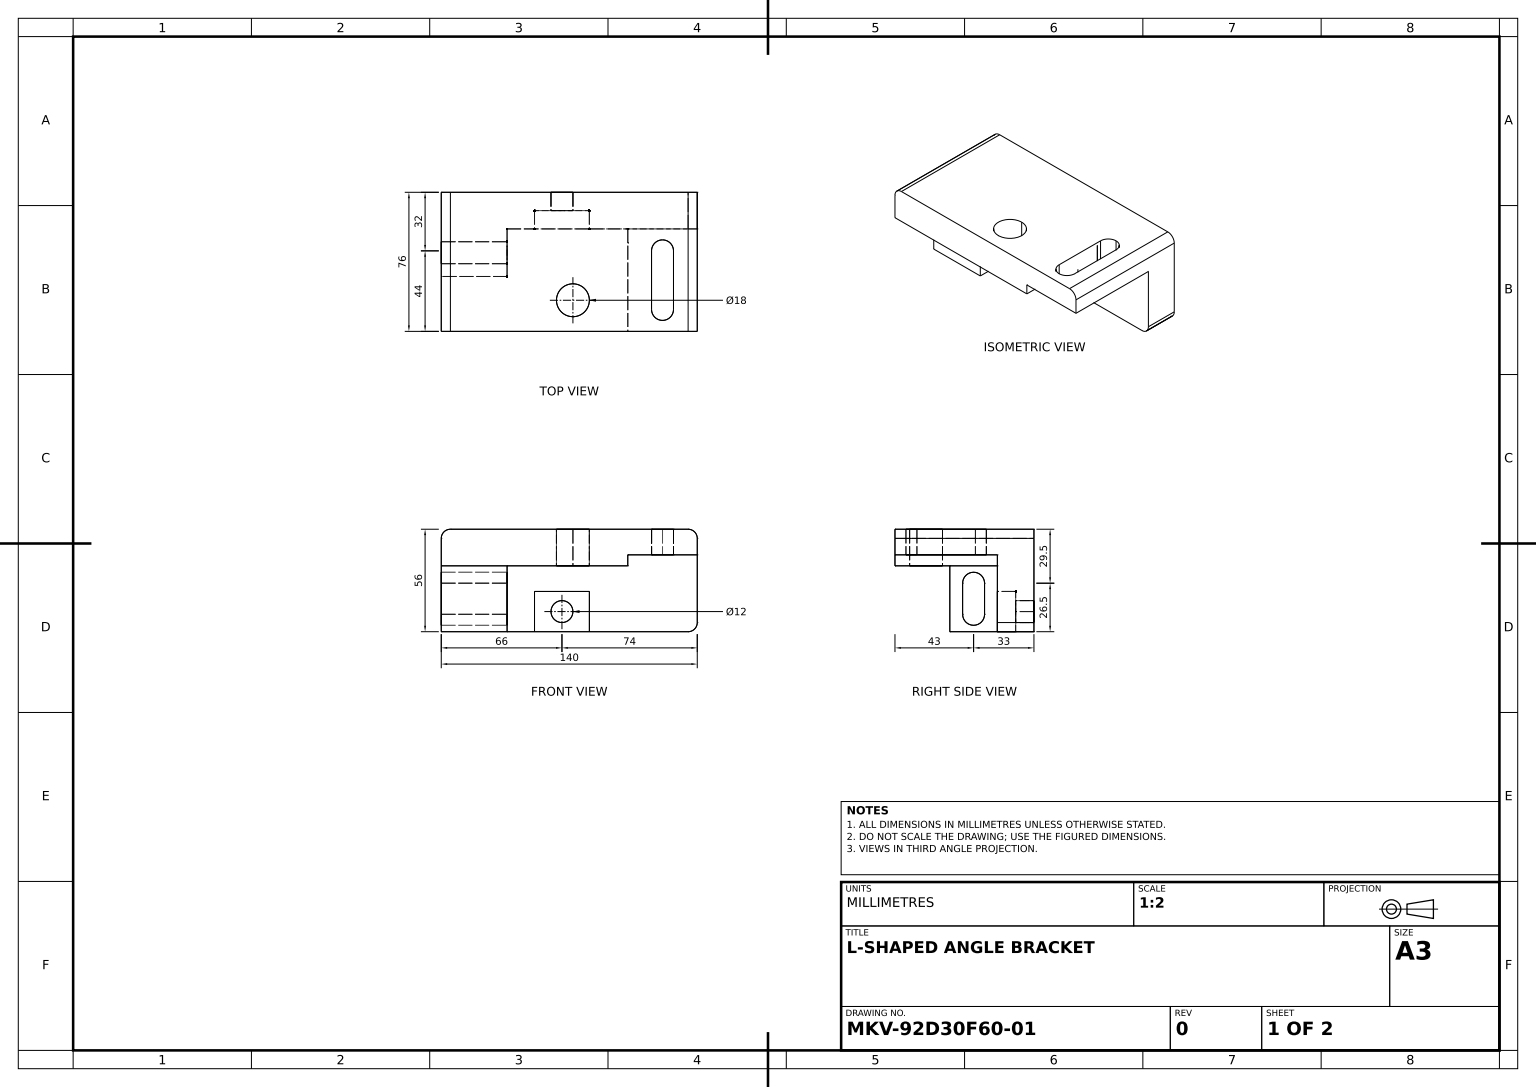
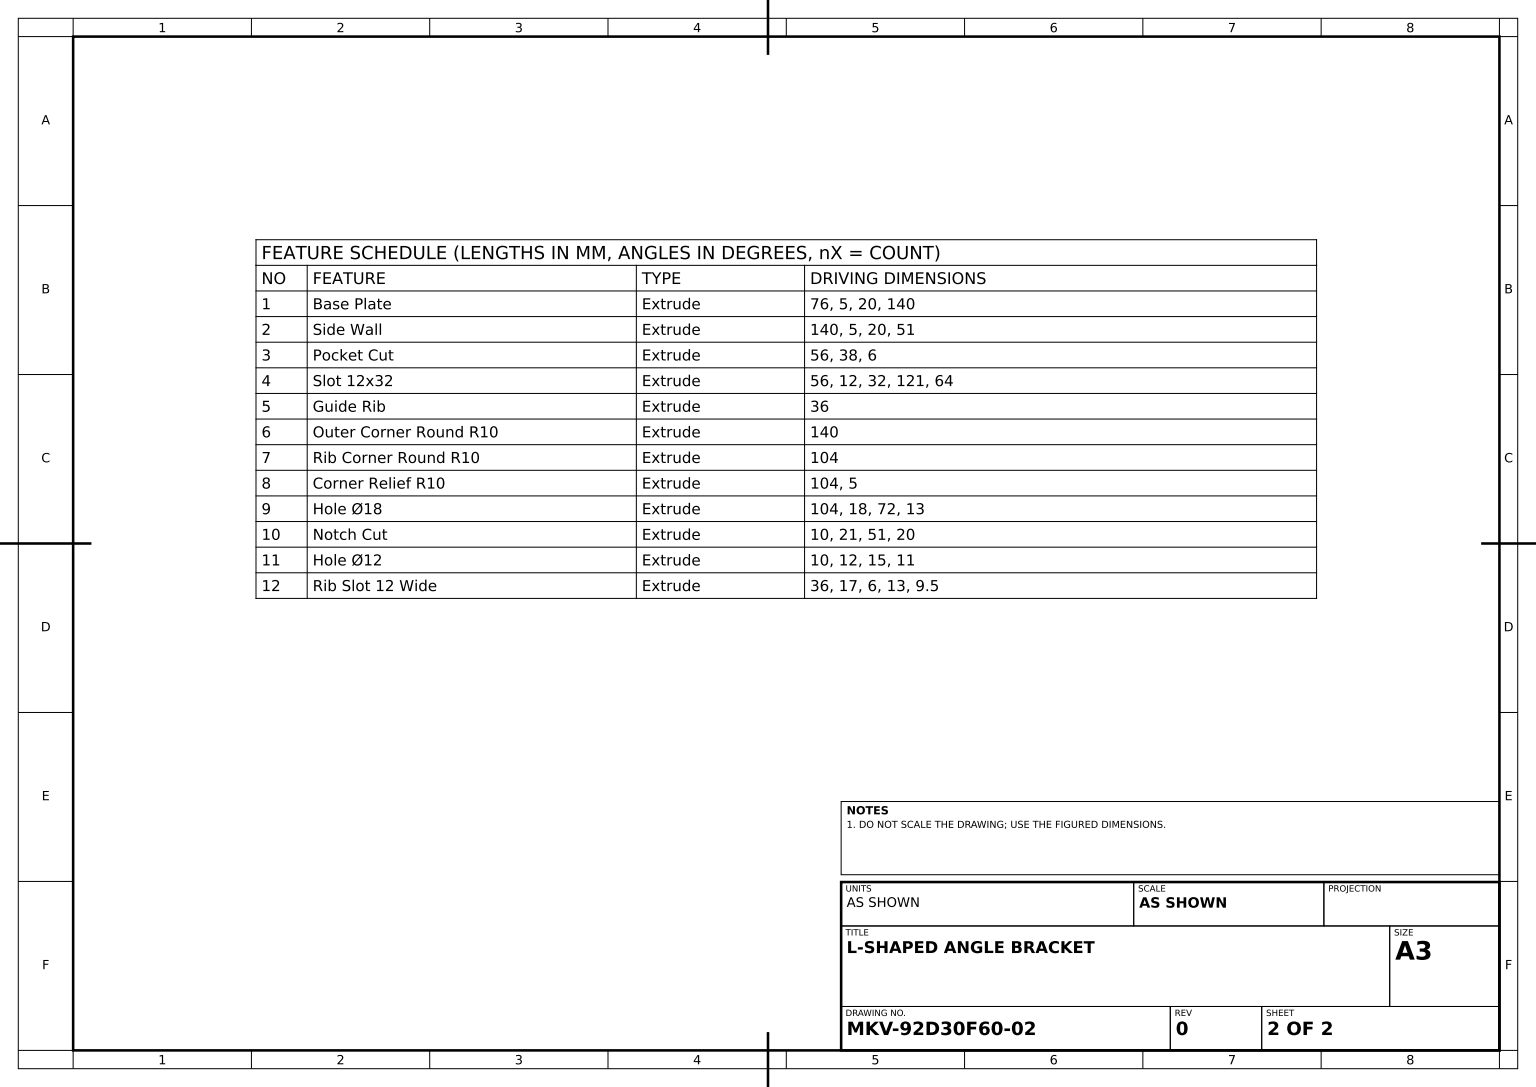
SolidWorks part; units mm, degrees
material "Plain Carbon Steel"
ref_plane "Front Plane" through (0, 0, 0) normal (0, 0, 1) x (1, 0, 0)
ref_plane "Top Plane" through (0, 0, 0) normal (0, 1, 0) x (1, 0, 0)
ref_plane "Right Plane" through (0, 0, 0) normal (1, 0, 0) x (0, 0, -1)
sketch "Base Plate Profile" plane through (0, 0, 0) normal (0, 0, 1) x (1, 0, 0)
  line L0 (5, 0) -> (135, 0)
  line L1 (140, -5) -> (140, -20)
  line L2 (140, -20) -> (0, -20)
  line L3 (0, -20) -> (0, -5)
  arc A0 (140, -5) -> (135, 0) centre (135, -5) ccw
  arc A1 (0, -5) -> (5, 0) centre (5, -5) cw
  point P9 (0, 0)
  dimension "D1" = 5
  dimension "D2" = 20
  dimension "D3" = 140
extrude "Base Plate" add sketch "Base Plate Profile" along normal blind 76
sketch "Side Wall Profile" plane through (140, 0, 0) normal (1, 0, 0) x (0, 0, -1)
  line L0 (0, -20) -> (0, -51)
  line L1 (-5, -56) -> (-15, -56)
  line L2 (-20, -51) -> (-20, -20)
  line L3 (-76, -20) -> (0, -20) construction
  line L4 (-20, -20) -> (0, -20)
  line L5 (-76, -5) -> (0, -5) construction
  arc A0 (-5, -56) -> (0, -51) centre (-5, -51) ccw
  arc A1 (-15, -56) -> (-20, -51) centre (-15, -51) cw
  dimension "D1" = 5
  dimension "D2" = 20
  dimension "D3" = 51
extrude "Side Wall" add sketch "Side Wall Profile" against normal blind 140
sketch "Pocket Profile" plane through (0, 0, 76) normal (0, 0, 1) x (1, 0, 0)
  line L0 (140, -20) -> (140, -14)
  line L1 (140, -20) -> (140, -5) construction
  line L2 (140, -14) -> (102, -14)
  line L3 (102, -14) -> (102, -20)
  line L4 (0, -20) -> (140, -20) construction
  line L5 (102, -20) -> (140, -20)
  line L6 (0, -20) -> (140, -20) construction
  dimension "D1" = 38
  dimension "D2" = 6
extrude "Pocket Cut" cut sketch "Pocket Profile" against normal blind 56
sketch "Slot 12x32 Profile" plane through (0, -14, 0) normal (0, -1, 0) x (1, 0, 0)
  line L4 (115, 64) -> (115, 32)
  line L5 (127, 64) -> (127, 32)
  arc A0 (127, 64) -> (115, 64) centre (121, 64) ccw
  arc A1 (115, 32) -> (127, 32) centre (121, 32) ccw
  dimension "D1" = 12
  dimension "D2" = 12
  dimension "D3" = 32
  dimension "D4" = 121
  dimension "D5" = 64
extrude "Slot 12x32" cut sketch "Slot 12x32 Profile" against normal blind 56
sketch "Guide Rib Profile" plane through (0, 0, 0) normal (-1, 0, 0) x (0, 0, 1)
  line L0 (20, -20) -> (46, -20)
  line L1 (76, -20) -> (20, -20) construction
  line L2 (46, -20) -> (46, -56)
  line L3 (46, -56) -> (15, -56)
  line L4 (20, -20) -> (20, -51)
  arc A0 (15, -56) -> (20, -51) centre (15, -51) ccw
  dimension "D1" = 10
extrude "Guide Rib" add sketch "Guide Rib Profile" against normal blind 36
sketch "Outer Corner Round Profile" plane through (0, 0, 0) normal (-1, 0, 0) x (0, 0, 1)
  line L0 (0, -51) -> (0, -56)
  line L1 (0, -56) -> (5, -56)
  arc A0 (0, -51) -> (5, -56) centre (5, -51) ccw
  dimension "D1" = 10
extrude "Outer Corner Round R10" add sketch "Outer Corner Round Profile" against normal blind 140
sketch "Rib Corner Round Profile" plane through (140, 0, 0) normal (1, 0, 0) x (0, 0, -1)
  line L0 (-20, -51) -> (-20, -56)
  line L1 (-20, -14) -> (-20, -51) construction
  line L2 (-15, -56) -> (-46, -56) construction
  line L3 (-20, -56) -> (-15, -56)
  arc A0 (-20, -51) -> (-15, -56) centre (-15, -51) ccw construction
  arc A1 (-20, -51) -> (-15, -56) centre (-15, -51) ccw
  dimension "D1" = 10
extrude "Rib Corner Round R10" add sketch "Rib Corner Round Profile" against normal blind 104
sketch "Corner Relief Profile" plane through (0, 0, 20) normal (0, 0, 1) x (1, 0, 0)
  line L0 (140, -56) -> (140, -51)
  line L1 (140, -14) -> (140, -56) construction
  line L3 (135, -56) -> (140, -56)
  arc A0 (135, -56) -> (140, -51) centre (135, -51) ccw
  dimension "D1" = 10
  dimension "D2" = 5
extrude "Corner Relief R10" cut sketch "Corner Relief Profile" against normal blind 104
sketch "Hole Ø18 Sketch" plane through (0, -20, 0) normal (0, -1, 0) x (1, 0, 0)
  line L0 (0, 76) -> (0, 46) construction
  line L1 (36, 46) -> (0, 46) construction
  circle A0 centre (72, 59) radius 9
  dimension "D1" = 18
  dimension "D2" = 72
  dimension "D3" = 13
extrude "Hole Ø18" cut sketch "Hole Ø18 Sketch" against normal blind 104
sketch "Notch Profile" plane through (0, 0, 20) normal (0, 0, 1) x (1, 0, 0)
  line L0 (102, -14) -> (102, -20) construction
  line L1 (36, -56) -> (135, -56) construction
  line L2 (51, -56) -> (51, -34)
  line L3 (51, -34) -> (81, -34)
  line L4 (81, -34) -> (81, -56)
  line L5 (81, -56) -> (51, -56)
  line L6 (140, -14) -> (102, -14) construction
  dimension "D1" = 21
  dimension "D2" = 51
  dimension "D3" = 20
extrude "Notch Cut" cut sketch "Notch Profile" against normal blind 10
sketch "Hole Ø12 Sketch" plane through (0, 0, 10) normal (0, 0, 1) x (1, 0, 0)
  line L0 (81, -56) -> (81, -34) construction
  line L1 (51, -56) -> (81, -56) construction
  circle A0 centre (66, -45) radius 6
  dimension "D1" = 12
  dimension "D2" = 12
  dimension "D3" = 15
  dimension "D4" = 11
extrude "Hole Ø12" cut sketch "Hole Ø12 Sketch" against normal blind 10
sketch "Rib Slot Profile" plane through (36, 0, 0) normal (1, 0, 0) x (0, 0, -1)
  line L0 (-20, -20) -> (-20, -56) construction
  line L1 (-20, -56) -> (-46, -56) construction
  line L4 (-39, -29.5) -> (-39, -46.5)
  line L5 (-27, -29.5) -> (-27, -46.5)
  arc A0 (-27, -29.5) -> (-39, -29.5) centre (-33, -29.5) ccw
  arc A1 (-39, -46.5) -> (-27, -46.5) centre (-33, -46.5) ccw
  dimension "D1" = 12
  dimension "D2" = 12
  dimension "D4" = 6
  dimension "D3" = 17
  dimension "D5" = 13
  dimension "D6" = 9.5
extrude "Rib Slot 12 Wide" cut sketch "Rib Slot Profile" against normal blind 36
